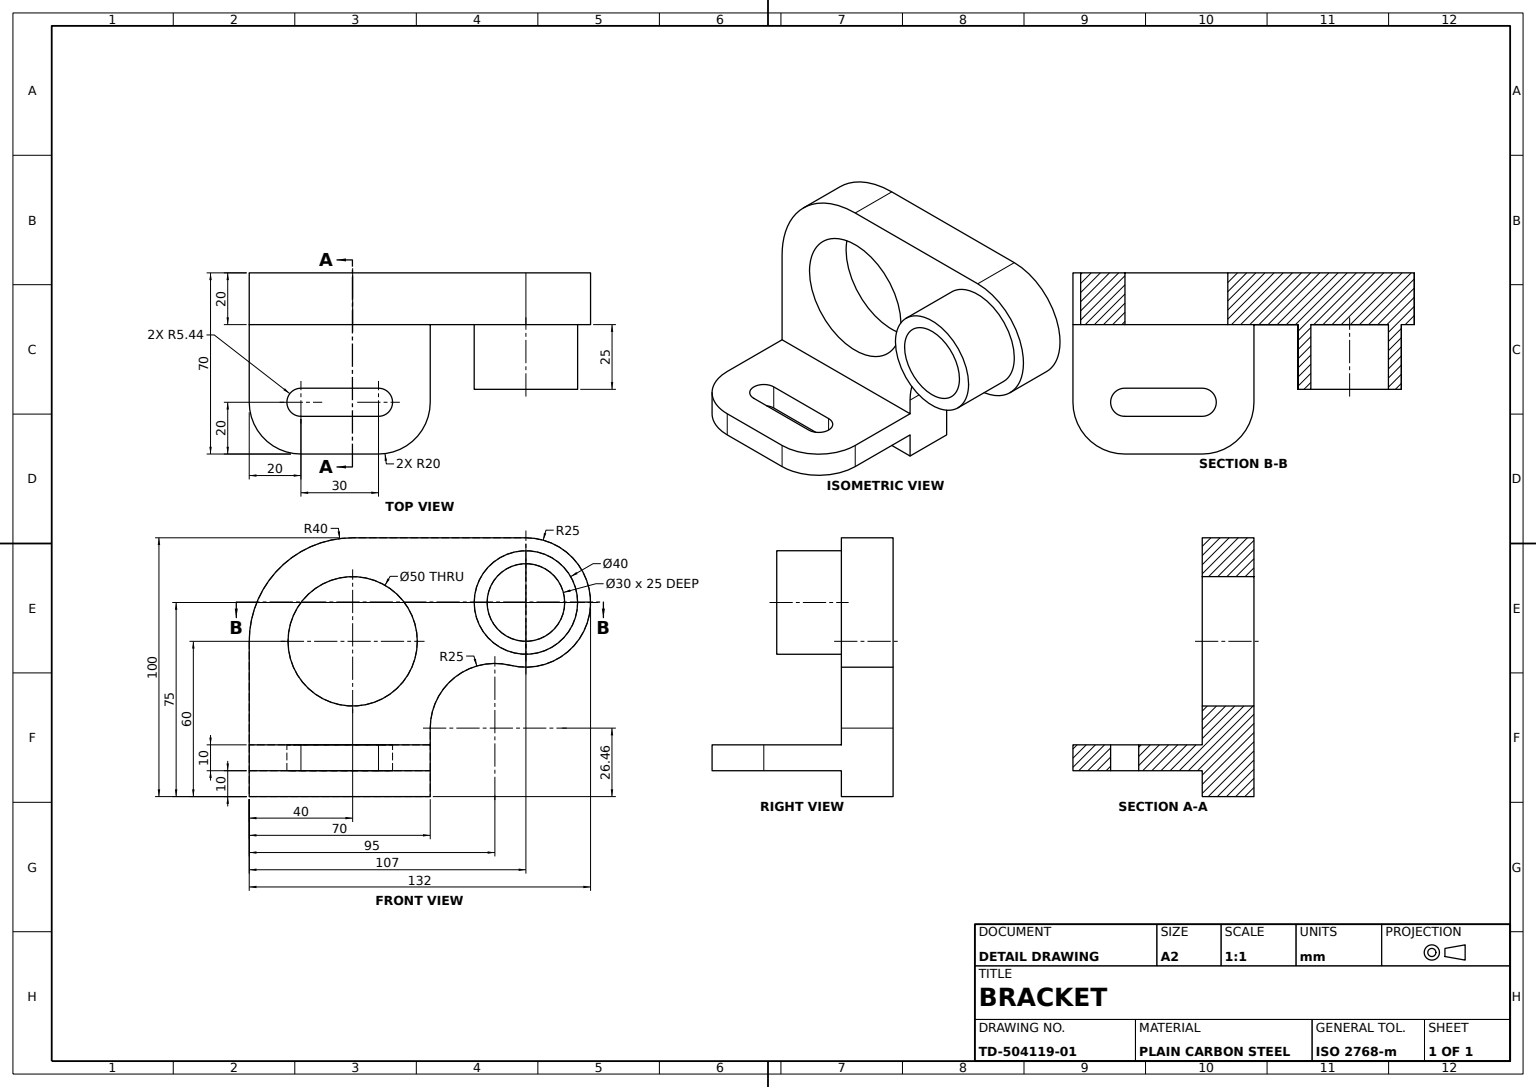
SolidWorks part; units mm, degrees
material "Plain Carbon Steel"
ref_plane "Front Plane" through (0, 0, 0) normal (0, 0, 1) x (1, 0, 0)
ref_plane "Top Plane" through (0, 0, 0) normal (0, 1, 0) x (1, 0, 0)
ref_plane "Right Plane" through (0, 0, 0) normal (1, 0, 0) x (0, 0, -1)
sketch "Upright Plate Profile" plane through (0, 0, 0) normal (0, 0, 1) x (1, 0, 0)
  line L1 (0, 0) -> (70, 0)
  line L3 (40, 100) -> (107, 100)
  line L4 (0, 0) -> (0, 60)
  line L11 (70, 26.4614) -> (70, 0)
  arc A2 (101, 50.7307) -> (107, 100) centre (107, 75) ccw
  arc A3 (70, 26.4614) -> (101, 50.7307) centre (95, 26.4614) cw
  arc A4 (0, 60) -> (40, 100) centre (40, 60) cw
  dimension "D1" = 70
  dimension "D3" = 40
  dimension "D4" = 25
  dimension "D5" = 25
  dimension "D2" = 100
  dimension "D6" = 107
extrude "Upright Plate" add sketch "Upright Plate Profile" along normal blind 20
sketch "Bearing Boss Profile" plane through (0, 0, 20) normal (0, 0, 1) x (1, 0, 0)
  circle A0 centre (107, 75) radius 15
  circle A1 centre (107, 75) radius 20
  dimension "D1" = 30
  dimension "D2" = 40
extrude "Bearing Boss" add sketch "Bearing Boss Profile" along normal blind 25
sketch "Bearing Bore Sketch" plane through (0, 0, 20) normal (0, 0, 1) x (1, 0, 0)
  circle A0 centre (40, 60) radius 25
  dimension "D1" = 50
extrude "Bearing Bore Ø50" cut sketch "Bearing Bore Sketch" against normal through all
ref_plane "Base Plate Offset Plane" through (0, 0, 20) normal (0, 0, 1) x (1, 0, 0)
sketch "Base Plate Profile" plane through (0, 0, 20) normal (0, 0, 1) x (1, 0, 0)
  line L1 (0, 20) -> (70, 20)
  line L2 (0, 20) -> (0, 10)
  line L3 (0, 10) -> (70, 10)
  line L4 (70, 20) -> (70, 10)
  line L5 (0, 20) -> (70, 10) construction
  line L6 (0, 10) -> (70, 20) construction
  line L8 (0, 60) -> (0, 0) construction
  line L9 (70, 0) -> (70, 26.4614) construction
  line L10 (0, 0) -> (70, 0) construction
  point P0 (35, 15)
  dimension "D1" = 10
  dimension "D2" = 10
extrude "Base Plate" add sketch "Base Plate Profile" along normal blind 50
fillet "Base Plate Corner Fillets R20" radius 20 2 edges at (0, 15, 70) (70, 15, 70)
sketch "Mounting Slot Sketch" plane through (0, 20, 0) normal (0, 1, 0) x (1, 0, 0)
  line L0 (20, -50) -> (50, -50) construction
  line L1 (20, -44.5647) -> (50, -44.5647)
  line L2 (20, -55.4353) -> (50, -55.4353)
  line L3 (0, -50) -> (0, -20) construction
  line L6 (50, -70) -> (20, -70) construction
  arc A0 (20, -44.5647) -> (20, -55.4353) centre (20, -50) ccw
  arc A1 (50, -55.4353) -> (50, -44.5647) centre (50, -50) ccw
  point P2 (35, -50)
  dimension "D4" = 5.4353
  dimension "D1" = 30
  dimension "D2" = 20
  dimension "D3" = 20
extrude "Mounting Slot" cut sketch "Mounting Slot Sketch" against normal through all
